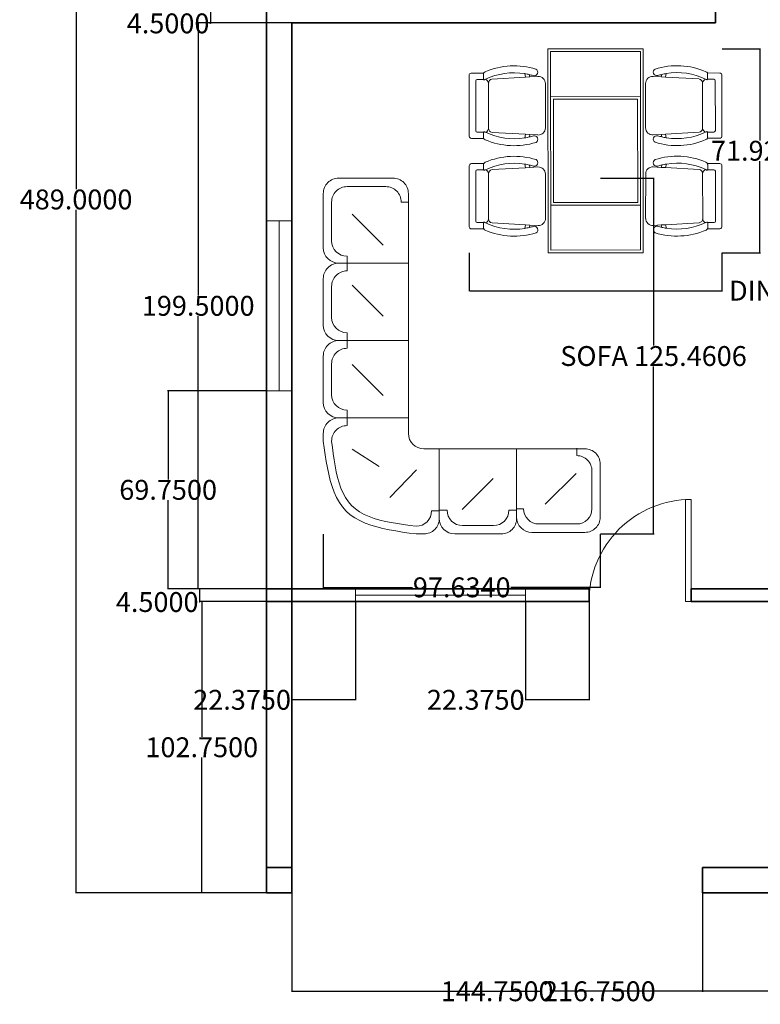
# Model space of a CAD drawing. Units: inches. Extents: x 774 to 2194, y 522 to 1247.
# Tile 1 of 7: x 774 to 1035, y 522 to 870. Entities that reach past the tile are written whole.
import ezdxf

# ---------------------------------------------------------------- set-up
doc = ezdxf.new("R2010")
doc.units = ezdxf.units.IN
for name, color, linetype, lineweight in [('A-ANNO-DIMS', 2, 'Continuous', 13), ('A-DOOR', 3, 'Continuous', 18), ('A-FURN', 8, 'Continuous', 18), ('A-GLAZ', 4, 'Continuous', 18), ('A-WALL', 7, 'Continuous', 35)]:
    doc.layers.add(name, color=color, linetype=linetype, lineweight=lineweight)
doc.styles.get("Standard").update_dxf_attribs({"font": 'arial.ttf'})
doc.dimstyles.get("Standard").update_dxf_attribs({"dimtxt": 7, "dimasz": 0.18, "dimexe": 0.18, "dimexo": 0.0625, "dimgap": 0.09, "dimtad": 0, "dimtih": 1, "dimtoh": 1, "dimdec": 4, "dimzin": 0, "dimdsep": 46, "dimtxsty": 'Standard', "dimcen": 0.09, "dimadec": 0, "dimazin": 0, "dimtfac": 1, "dimtdec": 4, "dimtofl": 0, "dimtmove": 0, "dimatfit": 3, "dimfxl": 1, "dimtolj": 1, "dimtzin": 0, "dimarcsym": 0})

# ---------------------------------------------------------------- blocks, each defined once
blk = doc.blocks.new('A$C7D96336B')
for p, q in [((280, 0.2), (-280, -0.2)), ((280.8, -1199.8), (280, 0.2)), ((-280, -0.2), (-279.2, -1200.2)), ((264, -15.8), (-264, -16.2)), ((-264, -16.2), (-263.2, -1184.2)), ((264.8, -1183.8), (264, -15.8)), ((-742.8, -515.1), (-743.2, -156.2)), ((-658.1, -143.4), (-730.7, -143.6)), ((-659.8, -143.4), (-659.7, -178.7)), ((-411.5, -167.3), (-609.1, -178.7)), ((-416.5, -146.3), (-411.5, -167.3)), ((-386.1, -165.8), (-411.5, -167.3)), ((-389.5, -151.7), (-386.1, -165.8)), ((-338.9, -163.1), (-386.1, -165.8)), ((339.1, -162.6), (386.3, -165.3)), ((389.7, -151.1), (386.3, -165.3)), ((386.3, -165.3), (411.7, -166.7)), ((416.7, -145.7), (411.7, -166.7)), ((411.7, -166.7), (609.3, -177.8)), ((658.3, -142.5), (730.9, -142.6)), ((659.9, -142.6), (659.9, -177.8)), ((743.5, -514.1), (743.4, -155.2)), ((-704.9, -188.8), (-704.6, -482.3)), ((-659.3, -180.3), (-696.6, -180.5)), ((-629.9, -467.6), (-630.2, -203.4)), ((-294.5, -465.7), (-294.4, -204.7)), ((295.2, -465.3), (294.7, -204.3)), ((630.5, -466.8), (630.5, -202.5)), ((659.5, -179.5), (696.9, -179.5)), ((705.2, -187.9), (705.3, -481.4)), ((-263.8, -280.2), (264.2, -279.8)), ((-263.8, -280.2), (264.2, -279.8)), ((-263.4, -920.2), (-263.8, -280.2)), ((264.2, -279.8), (264.6, -919.8)), ((-247.8, -296.2), (248.2, -295.8)), ((-247.4, -904.2), (-247.8, -296.2)), ((248.2, -295.8), (248.6, -903.8)), ((-659, -490.7), (-696.3, -490.7)), ((-659.4, -522.3), (-659.3, -492.4)), ((-411.1, -503.3), (-608.7, -492.3)), ((-416.1, -524.3), (-411.1, -503.3)), ((-385.8, -504.7), (-411.1, -503.3)), ((-389.1, -518.8), (-385.8, -504.7)), ((-338.5, -507.3), (-385.8, -504.7)), ((339.2, -506.9), (386.5, -504.2)), ((386.5, -504.2), (411.8, -502.7)), ((389.8, -518.3), (386.5, -504.2)), ((411.8, -502.7), (609.4, -491.4)), ((416.8, -523.7), (411.8, -502.7)), ((659.6, -489.8), (697, -489.7)), ((660.1, -521.4), (660, -491.5)), ((-657.7, -527.6), (-730.3, -527.6)), ((658.4, -526.7), (731, -526.6)), ((-742.7, -688.4), (-742.6, -1047.3)), ((-657.6, -675.8), (-730.2, -675.9)), ((-659.3, -681), (-659.2, -711)), ((-416, -678.8), (-411, -699.8)), ((-389, -684.2), (-385.6, -698.3)), ((339.3, -695.2), (386.6, -697.8)), ((389.9, -683.7), (386.6, -697.8)), ((416.9, -678.2), (411.9, -699.2)), ((658.5, -674.9), (731.1, -674.9)), ((660.2, -680.2), (660.2, -710.1)), ((743.6, -687.4), (744, -1046.3)), ((-704.4, -1014.6), (-704.5, -721.1)), ((-658.8, -712.7), (-696.2, -712.8)), ((-629.7, -735.7), (-629.6, -1000)), ((-411, -699.8), (-608.6, -711)), ((-385.6, -698.3), (-411, -699.8)), ((-338.4, -695.6), (-385.6, -698.3)), ((-294.4, -737.1), (-293.9, -998.2)), ((295.3, -736.7), (295.2, -997.8)), ((386.6, -697.8), (411.9, -699.2)), ((411.9, -699.2), (609.5, -710.2)), ((630.7, -734.9), (631, -999.1)), ((659.8, -711.8), (697.1, -711.8)), ((705.8, -1013.7), (705.5, -720.2)), ((264.6, -919.8), (-263.4, -920.2)), ((248.6, -903.8), (-247.4, -904.2)), ((-658.7, -1023), (-696.1, -1023)), ((-659.1, -1059.9), (-659.1, -1024.7)), ((-410.9, -1035.8), (-608.5, -1024.6)), ((-415.9, -1056.8), (-410.9, -1035.8)), ((-385.5, -1037.2), (-410.9, -1035.8)), ((-388.9, -1051.4), (-385.5, -1037.2)), ((-338.3, -1039.9), (-385.5, -1037.2)), ((339.7, -1039.4), (386.9, -1036.7)), ((386.9, -1036.7), (412.3, -1035.2)), ((390.3, -1050.8), (386.9, -1036.7)), ((412.3, -1035.2), (609.9, -1023.8)), ((417.3, -1056.2), (412.3, -1035.2)), ((660.1, -1022.1), (697.4, -1022)), ((660.6, -1059), (660.5, -1023.8)), ((-657.5, -1059.9), (-730.1, -1059.9)), ((658.9, -1059), (731.5, -1058.9)), ((-279.2, -1200.2), (280.8, -1199.8)), ((-263.2, -1184.2), (264.8, -1183.8))]:
    blk.add_line(p, q)
for centre, radius, start, end in [((-478.6, -532.7), 432.3, 72.71189, 113.32582), ((479.4, -532), 432.3, 66.7517, 107.36563), ((-730.7, -156.1), 12.5, 141.76048, 180.14594), ((-730.7, -156.1), 12.5, 90.1463, 141.76048), ((-643.2, -151), 16.7, 153.00405, 184.85665), ((-643.2, -151), 16.7, 113.32582, 153.00405), ((-479.1, -531.9), 390.7, 80.77031, 115.5809), ((-479.1, -531.9), 390.7, 76.73356, 80.77031), ((-479.1, -531.9), 390.7, 73.16759, 76.73356), ((-360.6, -137.9), 20.8, 254.77951, 60.01862), ((-336.5, -204.7), 41.7, 0.1463, 93.30684), ((336.7, -204.2), 41.7, 86.77068, 179.93121), ((360.7, -137.4), 20.8, 120.05889, 285.29801), ((479.9, -531.2), 390.7, 103.34395, 106.90992), ((479.9, -531.2), 390.7, 99.3072, 103.34395), ((479.9, -531.2), 390.7, 64.49661, 99.3072), ((643.4, -150.1), 16.7, 27.07347, 66.7517), ((643.4, -150.1), 16.7, 355.22086, 27.07347), ((730.9, -155.1), 12.5, 38.31704, 89.93121), ((730.9, -155.1), 12.5, 359.93158, 38.31704), ((-696.6, -188.8), 8.33, 90.1463, 180.1463), ((-655.5, -178.6), 4.17, 180.1463, 296.52957), ((-479.1, -531.9), 390.7, 115.5809, 116.52957), ((-655.2, -203.4), 25, 0.1463, 72.89681), ((-605.2, -203.4), 25, 98.92093, 179.97138), ((605.5, -202.6), 25, 0.10613, 81.15658), ((655.5, -202.5), 25, 107.1807, 179.93121), ((479.9, -531.2), 390.7, 63.54795, 64.49661), ((655.7, -177.8), 4.17, 243.54795, 359.93121), ((696.9, -187.8), 8.33, 359.93121, 89.93121), ((-730.3, -515.1), 12.5, 179.97174, 218.3572), ((-696.3, -482.3), 8.33, 179.97138, 269.97138), ((-642.9, -520), 16.7, 175.26103, 207.11363), ((-655.2, -492.4), 4.17, 63.58811, 179.97138), ((-479.5, -138.8), 390.7, 243.58811, 244.53678), ((-654.9, -467.6), 25, 287.22087, 359.97138), ((-479.5, -138.8), 390.7, 244.53678, 279.34737), ((-604.9, -467.6), 25, 180.1463, 261.19675), ((-479.5, -138.8), 390.7, 279.34737, 283.38411), ((-479.5, -138.8), 390.7, 283.38411, 286.95009), ((-360.2, -532.5), 20.8, 300.09905, 105.33817), ((-336.2, -465.7), 41.7, 266.81084, 359.97138), ((336.8, -465.3), 41.7, 180.10613, 273.26667), ((360.9, -532), 20.8, 74.73934, 239.97846), ((479.7, -138.1), 390.7, 253.12743, 256.6934), ((479.7, -138.1), 390.7, 256.6934, 260.73015), ((479.7, -138.1), 390.7, 260.73015, 295.54074), ((605.5, -466.7), 25, 278.88077, 359.93121), ((655.5, -466.7), 25, 180.10613, 252.85665), ((479.7, -138.1), 390.7, 295.54074, 296.4894), ((655.8, -491.5), 4.17, 0.10613, 116.4894), ((643.6, -519.1), 16.7, 332.96388, 4.81649), ((697, -481.4), 8.33, 270.10613, 0.10613), ((731, -514.1), 12.5, 321.72031, 0.10577), ((-730.3, -515.1), 12.5, 218.3572, 269.97138), ((-642.9, -520), 16.7, 207.11363, 246.79186), ((-479.1, -138), 432.3, 246.79186, 287.40579), ((479.2, -137.3), 432.3, 252.67172, 293.28565), ((643.6, -519.1), 16.7, 293.28565, 332.96388), ((731, -514.1), 12.5, 270.10613, 321.72031), ((-478.4, -1065.1), 432.3, 72.67172, 113.28565), ((479.9, -1064.5), 432.3, 66.79186, 107.40579), ((-730.2, -688.4), 12.5, 141.72031, 180.10577), ((-730.2, -688.4), 12.5, 90.10613, 141.72031), ((-642.7, -683.3), 16.7, 152.96388, 184.81649), ((-642.7, -683.3), 16.7, 113.28565, 152.96388), ((-478.9, -1064.3), 390.7, 80.73015, 115.54074), ((-478.9, -1064.3), 390.7, 76.6934, 80.73015), ((-478.9, -1064.3), 390.7, 73.12743, 76.6934), ((-360.1, -670.4), 20.8, 254.73934, 59.97846), ((337, -736.8), 41.7, 86.81084, 179.97138), ((361, -670), 20.8, 120.09905, 285.33817), ((480.4, -1063.7), 390.7, 103.38411, 106.95009), ((480.4, -1063.7), 390.7, 99.34737, 103.38411), ((480.4, -1063.7), 390.7, 64.53678, 99.34737), ((643.7, -682.5), 16.7, 27.11363, 66.79186), ((643.7, -682.5), 16.7, 355.26103, 27.11363), ((731.1, -687.4), 12.5, 38.3572, 89.97138), ((731.1, -687.4), 12.5, 359.97174, 38.3572), ((-696.1, -721.1), 8.33, 90.10613, 180.10613), ((-655, -711), 4.17, 180.10613, 296.4894), ((-478.9, -1064.3), 390.7, 115.54074, 116.4894), ((-654.7, -735.8), 25, 0.10613, 72.85665), ((-604.7, -735.7), 25, 98.88077, 179.93121), ((-336, -737.2), 41.7, 0.10613, 93.26667), ((605.7, -734.9), 25, 0.1463, 81.19675), ((655.7, -734.9), 25, 107.22087, 179.97138), ((480.4, -1063.7), 390.7, 63.58811, 64.53678), ((656, -710.1), 4.17, 243.58811, 359.97138), ((697.1, -720.1), 8.33, 359.97138, 89.97138), ((-696.1, -1014.6), 8.33, 179.93121, 269.93121), ((-654.9, -1024.7), 4.17, 63.54795, 179.93121), ((-479.1, -671.2), 390.7, 243.54795, 244.49661), ((-654.6, -1000), 25, 287.1807, 359.93121), ((-479.1, -671.2), 390.7, 244.49661, 279.3072), ((-604.6, -999.9), 25, 180.10613, 261.15658), ((-335.9, -998.3), 41.7, 266.77068, 359.93121), ((337.3, -997.8), 41.7, 180.1463, 273.30684), ((480, -670.6), 390.7, 260.77031, 295.5809), ((606, -999.1), 25, 278.92093, 359.97138), ((656, -999.1), 25, 180.1463, 252.89681), ((480, -670.6), 390.7, 295.5809, 296.52957), ((656.3, -1023.8), 4.17, 0.1463, 116.52957), ((697.4, -1013.7), 8.33, 270.1463, 0.1463), ((-730.1, -1047.4), 12.5, 179.93158, 218.31704), ((-730.1, -1047.4), 12.5, 218.31704, 269.93121), ((-642.6, -1052.4), 16.7, 175.22086, 207.07347), ((-642.6, -1052.4), 16.7, 207.07347, 246.7517), ((-478.6, -670.4), 432.3, 246.7517, 287.36563), ((-479.1, -671.2), 390.7, 279.3072, 283.34395), ((-479.1, -671.2), 390.7, 283.34395, 286.90992), ((-359.9, -1065.1), 20.8, 300.05889, 105.29801), ((361.4, -1064.6), 20.8, 74.77951, 240.01862), ((479.5, -669.8), 432.3, 252.71189, 293.32582), ((480, -670.6), 390.7, 253.16759, 256.73356), ((480, -670.6), 390.7, 256.73356, 260.77031), ((644, -1051.5), 16.7, 293.32582, 333.00405), ((644, -1051.5), 16.7, 333.00405, 4.85665), ((731.5, -1046.4), 12.5, 270.1463, 321.76048), ((731.5, -1046.4), 12.5, 321.76048, 0.14594)]:
    blk.add_arc(centre, radius, start, end)
blk = doc.blocks.new('A$C4B324E0D')
for points in [[(-0.4032, -0.0374), (-0.3959, 0.0153), (-0.3883, 0.0678), (-0.3801, 0.1195), (-0.3709, 0.1704), (-0.3605, 0.22), (-0.3485, 0.2679), (-0.3346, 0.314), (-0.3185, 0.3579), (-0.2998, 0.3993), (-0.2783, 0.4378), (-0.2537, 0.4731), (-0.2255, 0.5049), (-0.1936, 0.5331), (-0.1583, 0.5578), (-0.1198, 0.5793), (-0.0785, 0.5979), (-0.0346, 0.614), (0.0115, 0.628), (0.0595, 0.64), (0.1091, 0.6504), (0.1599, 0.6595), (0.2117, 0.6678), (0.2641, 0.6753), (0.3168, 0.6826)], [(-0.3432, -0.0374), (-0.3369, 0.0114), (-0.3303, 0.0599), (-0.3232, 0.1078), (-0.3151, 0.1548), (-0.3059, 0.2006), (-0.2951, 0.2449), (-0.2826, 0.2874), (-0.2681, 0.3278), (-0.2511, 0.3658), (-0.2315, 0.4011), (-0.2089, 0.4335), (-0.1831, 0.4625), (-0.1538, 0.488), (-0.1214, 0.5102), (-0.086, 0.5294), (-0.0479, 0.546), (-0.0075, 0.5602), (0.035, 0.5722), (0.0793, 0.5825), (0.125, 0.5914), (0.172, 0.599), (0.2198, 0.6057), (0.2682, 0.6119), (0.3168, 0.6177)], [(0.3768, 0.6826), (0.3168, 0.6826)], [(0.3168, 0.6177), (0.3168, 0.6177)], [(0.9768, 0.6826), (0.6168, 0.6826)], [(0.9168, 0.6177), (0.6768, 0.6177)], [(1.5769, 0.6826), (1.2168, 0.6826)], [(1.5168, 0.6177), (1.2768, 0.6177)], [(1.8168, 0.6826), (2.2368, 0.6826)], [(2.1704, 0.6177), (1.8704, 0.6177)], [(0.4968, 0.0226), (0.4968, 0.5626)], [(0.4968, 0.5626), (0.4968, 0.0226), (1.0968, 0.0226)], [(1.0968, 0.5626), (1.0968, 0.0226), (1.6968, 0.0226)], [(1.0968, 0.0226), (1.0968, 0.5626)], [(1.6968, 0.0226), (1.6968, 0.5626)], [(2.2368, 0.0226), (1.6968, 0.0226), (1.6968, 0.5626)], [(2.3569, 0.5626), (2.3569, 0.1426)], [(0.4968, 0.4977), (0.4368, 0.4977), (0.4368, 0.4977)], [(0.5569, 0.4977), (0.5569, 0.4977), (0.4968, 0.4977)], [(1.0968, 0.4977), (1.0368, 0.4977), (1.0368, 0.4977)], [(1.1569, 0.4977), (1.1569, 0.4977), (1.0968, 0.4977)], [(1.6969, 0.4977), (1.6368, 0.4977), (1.6368, 0.4977)], [(1.7504, 0.4977), (1.7504, 0.4977), (1.6904, 0.4977)], [(2.2904, 0.1977), (2.2904, 0.4977)], [(0.255, 0.4573), (0.1211, 0.2495)], [(0.9111, 0.4573), (0.6711, 0.2173)], [(1.527, 0.4573), (1.287, 0.2173)], [(2.0759, 0.4573), (1.8359, 0.2173)], [(-0.1199, 0.1664), (0.0943, -0.0414)], [(2.1704, 0.0177), (2.1704, 0.0777), (2.1704, 0.0777)], [(0.4968, 0.0226), (0.3768, 0.0226)], [(-0.4032, -0.0974), (-0.4032, -0.0374)], [(-0.3432, -0.0374), (-0.3432, -0.0374)], [(0.2568, -0.0974), (0.2568, -0.2174)], [(-0.2832, -0.8174), (0.2568, -0.8174), (0.2568, -0.2174)], [(0.2568, -0.2174), (-0.2832, -0.2174)], [(0.2568, -0.2174), (-0.2832, -0.2174)], [(-0.2232, -0.2174), (-0.2232, -0.1574), (-0.2232, -0.1574)], [(-0.2183, -0.2174), (-0.2183, -0.2774), (-0.2183, -0.2774)], [(-0.4032, -0.3374), (-0.4032, -0.6974)], [(-0.3383, -0.3974), (-0.3383, -0.6374)], [(-0.2136, -0.3946), (0.0264, -0.6346)], [(-0.2183, -0.7574), (-0.2183, -0.7574), (-0.2183, -0.8174)], [(0.2568, -0.8174), (-0.2832, -0.8174)], [(-0.2732, -0.8174), (0.2568, -0.8174), (0.2568, -1.3475)], [(-0.208, -0.8126), (-0.208, -0.8715), (-0.208, -0.8715)], [(0.2568, -0.8174), (0.2568, -1.3475)], [(-0.391, -1.3475), (-0.391, -0.9352)], [(-0.3258, -0.9893), (-0.3258, -1.2838)], [(-0.1734, -1.0387), (0.0666, -1.2787)], [(0.2043, -1.2838), (0.2043, -1.2838), (0.2632, -1.2838)], [(-0.208, -1.4016), (0.0865, -1.4016)], [(0.1391, -1.4653), (-0.2732, -1.4653)]]:
    blk.add_lwpolyline(points)
for centre, radius, start, end in [((0.3168, 0.4977), 0.12, 0, 90), ((0.3768, 0.5626), 0.12, 0, 90), ((0.6168, 0.5626), 0.12, 90, 180), ((0.6768, 0.4977), 0.12, 90, 180), ((0.9168, 0.4977), 0.12, 0, 90), ((0.9768, 0.5626), 0.12, 0, 90), ((1.2168, 0.5626), 0.12, 90, 180), ((1.2768, 0.4977), 0.12, 90, 180), ((1.5168, 0.4977), 0.12, 0, 90), ((1.5769, 0.5626), 0.12, 0, 90), ((1.8168, 0.5626), 0.12, 90, 180), ((1.8704, 0.4977), 0.12, 90, 180), ((2.1704, 0.4977), 0.12, 0, 90), ((2.2368, 0.5626), 0.12, 0, 90), ((2.1704, 0.1977), 0.12, 270, 0), ((2.2368, 0.1426), 0.12, 270, 0), ((0.3768, -0.0974), 0.12, 90, 180), ((-0.2232, -0.0374), 0.12, 180, 270), ((-0.2832, -0.0974), 0.12, 179.9997, 270), ((-0.2832, -0.3374), 0.12, 90, 180), ((-0.2183, -0.3974), 0.12, 90, 180), ((-0.2183, -0.6374), 0.12, 180, 270), ((-0.2832, -0.6974), 0.12, 179.9997, 270), ((-0.2732, -0.9352), 0.1178, 90, 180), ((-0.208, -0.9893), 0.1178, 90, 180), ((-0.208, -1.2838), 0.1178, 180, 270), ((0.0865, -1.2838), 0.1178, 270, 0), ((-0.2732, -1.3475), 0.1178, 179.9997, 270), ((0.1391, -1.3475), 0.1178, 270, 0)]:
    blk.add_arc(centre, radius, start, end)
blk = doc.blocks.new('A$C58C6152E')
at = {"xscale": 1.5, "yscale": 1.5, "zscale": 1.5, "rotation": 90}
blk.add_blockref('A$C4B324E0D', (1.024, 0.605), dxfattribs=at)
blk = doc.blocks.new('A$C15DC316E')
at = {"xscale": -1, "rotation": 270}
blk.add_blockref('A$C58C6152E', (0, 0), dxfattribs=at)
blk = doc.blocks.new('*D18')
at = {"layer": 'A-ANNO-DIMS', "color": 0, "lineweight": -2, "transparency": 16777216}
for p, q in [((869.72, 872.94), (840.87, 872.94)), ((841.05, 872.76), (841.05, 868.62)), ((869.72, 868.44), (840.87, 868.44)), ((841.05, 868.26), (840.87, 868.26)), ((841.05, 868.44), (841.05, 868.26))]:
    blk.add_line(p, q, dxfattribs=at)
at = {"layer": 'A-ANNO-DIMS', "color": 0, "transparency": 16777216}
for points in [[(841.02, 872.76), (841.08, 872.76), (841.05, 872.94)], [(841.02, 868.62), (841.08, 868.62), (841.05, 868.44)]]:
    blk.add_solid(points, dxfattribs=at)
at = {"layer": 'Defpoints', "color": 0, "transparency": 16777216}
for p in [(869.78, 872.94), (841.05, 868.44), (869.78, 868.44)]:
    blk.add_point(p, dxfattribs=at)
at = {"layer": 'A-ANNO-DIMS', "color": 0, "transparency": 16777216, "insert": (826.12, 868.26), "char_height": 7, "attachment_point": 5}
blk.add_mtext('\\A1;4.5000', dxfattribs=at)
blk = doc.blocks.new('*D19')
at = {"layer": 'A-ANNO-DIMS', "color": 0, "lineweight": -2, "transparency": 16777216}
for p, q in [((869.72, 868.44), (836.55, 868.44)), ((836.73, 868.26), (836.73, 772.35)), ((836.73, 669.12), (836.73, 765.02)), ((869.72, 668.94), (836.55, 668.94))]:
    blk.add_line(p, q, dxfattribs=at)
at = {"layer": 'A-ANNO-DIMS', "color": 0, "transparency": 16777216}
for points in [[(836.7, 868.26), (836.76, 868.26), (836.73, 868.44)], [(836.7, 669.12), (836.76, 669.12), (836.73, 668.94)]]:
    blk.add_solid(points, dxfattribs=at)
at = {"layer": 'Defpoints', "color": 0, "transparency": 16777216}
for p in [(869.78, 868.44), (836.73, 668.94), (869.78, 668.94)]:
    blk.add_point(p, dxfattribs=at)
at = {"layer": 'A-ANNO-DIMS', "color": 0, "transparency": 16777216, "insert": (836.73, 768.69), "char_height": 7, "attachment_point": 5}
blk.add_mtext('\\A1;199.5000', dxfattribs=at)
blk = doc.blocks.new('*D20')
at = {"layer": 'A-ANNO-DIMS', "color": 0, "lineweight": -2, "transparency": 16777216}
for p, q in [((869.72, 668.94), (837.03, 668.94)), ((837.21, 668.76), (837.21, 664.62)), ((869.72, 664.44), (837.03, 664.44)), ((837.21, 664.26), (837.03, 664.26)), ((837.21, 664.44), (837.21, 664.26))]:
    blk.add_line(p, q, dxfattribs=at)
at = {"layer": 'A-ANNO-DIMS', "color": 0, "transparency": 16777216}
for points in [[(837.18, 668.76), (837.24, 668.76), (837.21, 668.94)], [(837.18, 664.62), (837.24, 664.62), (837.21, 664.44)]]:
    blk.add_solid(points, dxfattribs=at)
at = {"layer": 'Defpoints', "color": 0, "transparency": 16777216}
for p in [(869.78, 668.94), (837.21, 664.44), (869.78, 664.44)]:
    blk.add_point(p, dxfattribs=at)
at = {"layer": 'A-ANNO-DIMS', "color": 0, "transparency": 16777216, "insert": (822.28, 664.26), "char_height": 7, "attachment_point": 5}
blk.add_mtext('\\A1;4.5000', dxfattribs=at)
blk = doc.blocks.new('*D21')
at = {"layer": 'A-ANNO-DIMS', "color": 0, "lineweight": -2, "transparency": 16777216}
for p, q in [((869.72, 664.44), (837.82, 664.44)), ((838, 664.26), (838, 616.73)), ((838, 561.87), (838, 609.4)), ((869.72, 561.69), (837.82, 561.69))]:
    blk.add_line(p, q, dxfattribs=at)
at = {"layer": 'A-ANNO-DIMS', "color": 0, "transparency": 16777216}
for points in [[(837.97, 664.26), (838.03, 664.26), (838, 664.44)], [(837.97, 561.87), (838.03, 561.87), (838, 561.69)]]:
    blk.add_solid(points, dxfattribs=at)
at = {"layer": 'Defpoints', "color": 0, "transparency": 16777216}
for p in [(869.78, 664.44), (838, 561.69), (869.78, 561.69)]:
    blk.add_point(p, dxfattribs=at)
at = {"layer": 'A-ANNO-DIMS', "color": 0, "transparency": 16777216, "insert": (838, 613.06), "char_height": 7, "attachment_point": 5}
blk.add_mtext('\\A1;102.7500', dxfattribs=at)
blk = doc.blocks.new('*D22')
at = {"layer": 'A-ANNO-DIMS', "color": 0, "lineweight": -2, "transparency": 16777216}
for p, q in [((869.72, 1050.69), (793.49, 1050.69)), ((793.67, 1050.51), (793.67, 809.85)), ((793.67, 561.87), (793.67, 802.52)), ((869.72, 561.69), (793.49, 561.69))]:
    blk.add_line(p, q, dxfattribs=at)
at = {"layer": 'A-ANNO-DIMS', "color": 0, "transparency": 16777216}
for points in [[(793.64, 1050.51), (793.7, 1050.51), (793.67, 1050.69)], [(793.64, 561.87), (793.7, 561.87), (793.67, 561.69)]]:
    blk.add_solid(points, dxfattribs=at)
at = {"layer": 'Defpoints', "color": 0, "transparency": 16777216}
for p in [(869.78, 1050.69), (793.67, 561.69), (869.78, 561.69)]:
    blk.add_point(p, dxfattribs=at)
at = {"layer": 'A-ANNO-DIMS', "color": 0, "transparency": 16777216, "insert": (793.67, 806.19), "char_height": 7, "attachment_point": 5}
blk.add_mtext('\\A1;489.0000', dxfattribs=at)
blk = doc.blocks.new('DOOR-SWING-36IN')
blk.add_line((36, 0), (36, 2))
blk.add_lwpolyline([(36, 2), (0, 2), (0, 0), (36, 0)], close=True)
blk.add_arc((36, 0), 36, 90, 180)
blk = doc.blocks.new('WIN-60IN-EXT')
for p, q in [((0, 0), (0, 9)), ((60, 0), (60, 9)), ((0, 4.5), (60, 4.5))]:
    blk.add_line(p, q)
blk = doc.blocks.new('*D46')
at = {"layer": 'A-ANNO-DIMS', "color": 0, "lineweight": -2, "transparency": 16777216}
for p, q in [((932.28, 787.34), (932.28, 773.85)), ((1021.39, 787.34), (1021.39, 773.85)), ((932.46, 774.03), (1021.21, 774.03)), ((1021.39, 774.03), (1021.57, 774.03))]:
    blk.add_line(p, q, dxfattribs=at)
at = {"layer": 'A-ANNO-DIMS', "color": 0, "transparency": 16777216}
for points in [[(932.46, 774.06), (932.46, 774), (932.28, 774.03)], [(1021.21, 774.06), (1021.21, 774), (1021.39, 774.03)]]:
    blk.add_solid(points, dxfattribs=at)
at = {"layer": 'Defpoints', "color": 0, "transparency": 16777216}
for p in [(932.28, 787.4), (1021.39, 787.4), (1021.39, 774.03)]:
    blk.add_point(p, dxfattribs=at)
at = {"layer": 'A-ANNO-DIMS', "color": 0, "transparency": 16777216, "insert": (1068.06, 774.03), "char_height": 7, "attachment_point": 5}
blk.add_mtext('\\A1;DINING SET 89.1080', dxfattribs=at)
blk = doc.blocks.new('*D47')
at = {"layer": 'A-ANNO-DIMS', "color": 0, "lineweight": -2, "transparency": 16777216}
for p, q in [((1021.45, 859.32), (1034.94, 859.32)), ((1034.76, 859.14), (1034.76, 827.02)), ((1034.76, 787.58), (1034.76, 819.7)), ((1021.45, 787.4), (1034.94, 787.4))]:
    blk.add_line(p, q, dxfattribs=at)
at = {"layer": 'A-ANNO-DIMS', "color": 0, "transparency": 16777216}
for points in [[(1034.73, 859.14), (1034.79, 859.14), (1034.76, 859.32)], [(1034.73, 787.58), (1034.79, 787.58), (1034.76, 787.4)]]:
    blk.add_solid(points, dxfattribs=at)
at = {"layer": 'Defpoints', "color": 0, "transparency": 16777216}
for p in [(1021.39, 859.32), (1034.76, 859.32), (1021.39, 787.4)]:
    blk.add_point(p, dxfattribs=at)
at = {"layer": 'A-ANNO-DIMS', "color": 0, "transparency": 16777216, "insert": (1034.76, 823.36), "char_height": 7, "attachment_point": 5}
blk.add_mtext('\\A1;71.9216', dxfattribs=at)
blk = doc.blocks.new('*D48')
at = {"layer": 'A-ANNO-DIMS', "color": 0, "lineweight": -2, "transparency": 16777216}
for p, q in [((978.53, 813.72), (997.46, 813.72)), ((997.28, 813.54), (997.28, 754.7)), ((997.28, 688.44), (997.28, 747.27)), ((978.53, 688.26), (997.46, 688.26))]:
    blk.add_line(p, q, dxfattribs=at)
at = {"layer": 'A-ANNO-DIMS', "color": 0, "transparency": 16777216}
for points in [[(997.25, 813.54), (997.31, 813.54), (997.28, 813.72)], [(997.25, 688.44), (997.31, 688.44), (997.28, 688.26)]]:
    blk.add_solid(points, dxfattribs=at)
at = {"layer": 'Defpoints', "color": 0, "transparency": 16777216}
for p in [(978.46, 813.72), (997.28, 813.72), (978.46, 688.26)]:
    blk.add_point(p, dxfattribs=at)
at = {"layer": 'A-ANNO-DIMS', "color": 0, "transparency": 16777216, "insert": (997.28, 750.99), "char_height": 7, "attachment_point": 5}
blk.add_mtext('\\A1;SOFA 125.4606', dxfattribs=at)
blk = doc.blocks.new('*D49')
at = {"layer": 'A-ANNO-DIMS', "color": 0, "lineweight": -2, "transparency": 16777216}
for p, q in [((880.83, 688.19), (880.83, 669.26)), ((978.46, 688.19), (978.46, 669.26)), ((881.01, 669.44), (912.32, 669.44)), ((978.28, 669.44), (946.97, 669.44))]:
    blk.add_line(p, q, dxfattribs=at)
at = {"layer": 'A-ANNO-DIMS', "color": 0, "transparency": 16777216}
for points in [[(881.01, 669.47), (881.01, 669.41), (880.83, 669.44)], [(978.28, 669.47), (978.28, 669.41), (978.46, 669.44)]]:
    blk.add_solid(points, dxfattribs=at)
at = {"layer": 'Defpoints', "color": 0, "transparency": 16777216}
for p in [(880.83, 688.26), (978.46, 688.26), (978.46, 669.44)]:
    blk.add_point(p, dxfattribs=at)
at = {"layer": 'A-ANNO-DIMS', "color": 0, "transparency": 16777216, "insert": (929.65, 669.44), "char_height": 7, "attachment_point": 5}
blk.add_mtext('\\A1;97.6340', dxfattribs=at)
blk = doc.blocks.new('*D54')
at = {"layer": 'A-ANNO-DIMS', "color": 0, "lineweight": -2, "transparency": 16777216}
for p, q in [((869.78, 561.63), (869.78, 526.86)), ((1014.53, 561.63), (1014.53, 526.86)), ((869.96, 527.04), (922.44, 527.04)), ((1014.35, 527.04), (961.87, 527.04))]:
    blk.add_line(p, q, dxfattribs=at)
at = {"layer": 'A-ANNO-DIMS', "color": 0, "transparency": 16777216}
for points in [[(869.96, 527.07), (869.96, 527.01), (869.78, 527.04)], [(1014.35, 527.07), (1014.35, 527.01), (1014.53, 527.04)]]:
    blk.add_solid(points, dxfattribs=at)
at = {"layer": 'Defpoints', "color": 0, "transparency": 16777216}
for p in [(869.78, 561.69), (1014.53, 561.69), (1014.53, 527.04)]:
    blk.add_point(p, dxfattribs=at)
at = {"layer": 'A-ANNO-DIMS', "color": 0, "transparency": 16777216, "insert": (942.16, 527.04), "char_height": 7, "attachment_point": 5}
blk.add_mtext('\\A1;144.7500', dxfattribs=at)
blk = doc.blocks.new('*D55')
at = {"layer": 'A-ANNO-DIMS', "color": 0, "lineweight": -2, "transparency": 16777216}
for p, q in [((869.78, 668.88), (869.78, 526.86)), ((1086.53, 668.88), (1086.53, 526.86)), ((869.96, 527.04), (958.05, 527.04)), ((1086.35, 527.04), (998.26, 527.04))]:
    blk.add_line(p, q, dxfattribs=at)
at = {"layer": 'A-ANNO-DIMS', "color": 0, "transparency": 16777216}
for points in [[(869.96, 527.07), (869.96, 527.01), (869.78, 527.04)], [(1086.35, 527.07), (1086.35, 527.01), (1086.53, 527.04)]]:
    blk.add_solid(points, dxfattribs=at)
at = {"layer": 'Defpoints', "color": 0, "transparency": 16777216}
for p in [(869.78, 668.94), (1086.53, 668.94), (1086.53, 527.04)]:
    blk.add_point(p, dxfattribs=at)
at = {"layer": 'A-ANNO-DIMS', "color": 0, "transparency": 16777216, "insert": (978.16, 527.04), "char_height": 7, "attachment_point": 5}
blk.add_mtext('\\A1;216.7500', dxfattribs=at)
blk = doc.blocks.new('*D56')
at = {"layer": 'A-ANNO-DIMS', "color": 0, "lineweight": -2, "transparency": 16777216}
for p, q in [((869.78, 664.38), (869.78, 629.61)), ((892.16, 664.38), (892.16, 629.61)), ((869.78, 629.79), (869.6, 629.79)), ((891.98, 629.79), (869.96, 629.79))]:
    blk.add_line(p, q, dxfattribs=at)
at = {"layer": 'A-ANNO-DIMS', "color": 0, "transparency": 16777216}
for points in [[(869.96, 629.82), (869.96, 629.76), (869.78, 629.79)], [(891.98, 629.82), (891.98, 629.76), (892.16, 629.79)]]:
    blk.add_solid(points, dxfattribs=at)
at = {"layer": 'Defpoints', "color": 0, "transparency": 16777216}
for p in [(869.78, 664.44), (892.16, 664.44), (869.78, 629.79)]:
    blk.add_point(p, dxfattribs=at)
at = {"layer": 'A-ANNO-DIMS', "color": 0, "transparency": 16777216, "insert": (852.21, 629.79), "char_height": 7, "attachment_point": 5}
blk.add_mtext('\\A1;22.3750', dxfattribs=at)
blk = doc.blocks.new('*D57')
at = {"layer": 'A-ANNO-DIMS', "color": 0, "lineweight": -2, "transparency": 16777216}
for p, q in [((952.16, 664.38), (952.16, 629.61)), ((974.53, 664.38), (974.53, 629.61)), ((952.16, 629.79), (951.98, 629.79)), ((974.35, 629.79), (952.34, 629.79))]:
    blk.add_line(p, q, dxfattribs=at)
at = {"layer": 'A-ANNO-DIMS', "color": 0, "transparency": 16777216}
for points in [[(952.34, 629.82), (952.34, 629.76), (952.16, 629.79)], [(974.35, 629.82), (974.35, 629.76), (974.53, 629.79)]]:
    blk.add_solid(points, dxfattribs=at)
at = {"layer": 'Defpoints', "color": 0, "transparency": 16777216}
for p in [(952.16, 664.44), (974.53, 664.44), (952.16, 629.79)]:
    blk.add_point(p, dxfattribs=at)
at = {"layer": 'A-ANNO-DIMS', "color": 0, "transparency": 16777216, "insert": (934.59, 629.79), "char_height": 7, "attachment_point": 5}
blk.add_mtext('\\A1;22.3750', dxfattribs=at)
blk = doc.blocks.new('*D62')
at = {"layer": 'A-ANNO-DIMS', "color": 0, "lineweight": -2, "transparency": 16777216}
for p, q in [((860.72, 738.69), (825.95, 738.69)), ((826.13, 738.51), (826.13, 707.48)), ((826.13, 669.12), (826.13, 700.15)), ((860.72, 668.94), (825.95, 668.94))]:
    blk.add_line(p, q, dxfattribs=at)
at = {"layer": 'A-ANNO-DIMS', "color": 0, "transparency": 16777216}
for points in [[(826.1, 738.51), (826.16, 738.51), (826.13, 738.69)], [(826.1, 669.12), (826.16, 669.12), (826.13, 668.94)]]:
    blk.add_solid(points, dxfattribs=at)
at = {"layer": 'Defpoints', "color": 0, "transparency": 16777216}
for p in [(826.13, 738.69), (860.78, 738.69), (860.78, 668.94)]:
    blk.add_point(p, dxfattribs=at)
at = {"layer": 'A-ANNO-DIMS', "color": 0, "transparency": 16777216, "insert": (826.13, 703.81), "char_height": 7, "attachment_point": 5}
blk.add_mtext('\\A1;69.7500', dxfattribs=at)

msp = doc.modelspace()

# ---------------------------------------------------------------- linework, layer by layer
at = {"layer": 'A-GLAZ'}
for p, q in [((892.15603, 664.4375), (892.15603, 668.9375)), ((892.15603, 666.6875), (952.15603, 666.6875)), ((952.15603, 664.4375), (952.15603, 668.9375))]:
    msp.add_line(p, q, dxfattribs=at)
at = {"layer": 'A-WALL'}
for p, q in [((860.78103, 1050.6875), (860.78103, 561.6875)), ((1019.07934, 872.9375), (1019.08056, 868.4375)), ((869.78103, 868.4375), (1019.08056, 868.4375)), ((869.78103, 868.4375), (869.78103, 668.9375)), ((869.78103, 868.4375), (869.78103, 561.6875)), ((860.78103, 668.9375), (974.53103, 668.9375)), ((974.53103, 664.4375), (974.53103, 668.9375)), ((1010.53103, 664.4375), (1010.53103, 668.9375)), ((1010.53103, 668.9375), (1086.53103, 668.9375)), ((860.78103, 664.4375), (974.53103, 664.4375)), ((869.78103, 664.4375), (974.53103, 664.4375)), ((1010.53103, 664.4375), (1211.78103, 664.4375)), ((860.78103, 570.6875), (869.78103, 570.6875)), ((1014.53103, 570.6875), (1014.53103, 561.6875)), ((1014.53103, 570.6875), (1211.78103, 570.6875)), ((860.78103, 561.6875), (869.78103, 561.6875)), ((1014.53103, 561.6875), (1220.78103, 561.6875))]:
    msp.add_line(p, q, dxfattribs=at)

# ---------------------------------------------------------------- block references
at = {"layer": 'A-DOOR', "extrusion": (0, 0, -1), "zscale": -1, "rotation": 270.0000000000003}
msp.add_blockref('DOOR-SWING-36IN', (-1010.53061, 700.43708), dxfattribs=at)
at = {"layer": 'A-FURN', "xscale": 0.0599157891524393, "yscale": 0.0599157891524393, "zscale": 0.0599157891524393}
msp.add_blockref('A$C7D96336B', (976.81224, 859.30902), dxfattribs=at)
at = {"layer": 'A-FURN', "xscale": -30.30437697783735, "yscale": 30.30437697783735, "zscale": 30.30437697783735, "rotation": 270}
msp.add_blockref('A$C15DC316E', (880.82882, 688.25576), dxfattribs=at)
at = {"layer": 'A-GLAZ', "rotation": 89.99999999999957}
msp.add_blockref('WIN-60IN-EXT', (869.78053, 738.68748), dxfattribs=at)

# ---------------------------------------------------------------- dimensions: what is measured, and where the dimension line sits
at = {"layer": 'A-ANNO-DIMS'}
for base, p1, p2, angle, override, picture, middle in [((793.67062, 561.6875), (869.78103, 1050.6875), (869.78103, 561.6875), 90, {"dimclrd": 0, "dimclre": 0, "dimclrt": 0}, '*D22', (793.67062, 806.1875)), ((841.05064, 868.4375), (869.78103, 872.9375), (869.78103, 868.4375), 90, {"dimclrd": 0, "dimclre": 0, "dimclrt": 0}, '*D18', (826.1217, 868.2575)), ((836.72755, 668.9375), (869.78103, 868.4375), (869.78103, 668.9375), 90, {"dimclrd": 0, "dimclre": 0, "dimclrt": 0}, '*D19', (836.72755, 768.6875)), ((1034.75683, 859.32037), (1021.39063, 787.39874), (1021.39063, 859.32037), 90, {"dimdec": 4, "dimlfac": 1, "dimrnd": 0, "dimzin": 0, "dimdsep": 46, "dimlunit": 2}, '*D47', (1034.75683, 823.35956)), ((826.13103, 738.6875), (860.78103, 668.9375), (860.78103, 738.6875), 90, {"dimdec": 4, "dimlfac": 1, "dimrnd": 0, "dimzin": 0, "dimdsep": 46, "dimlunit": 2}, '*D62', (826.13103, 703.8125)), ((837.20822, 664.4375), (869.78103, 668.9375), (869.78103, 664.4375), 90, {"dimclrd": 0, "dimclre": 0, "dimclrt": 0}, '*D20', (822.27928, 664.2575)), ((838.00015, 561.6875), (869.78103, 664.4375), (869.78103, 561.6875), 90, {"dimclrd": 0, "dimclre": 0, "dimclrt": 0}, '*D21', (838.00015, 613.0625)), ((869.78103, 629.7875), (892.15603, 664.4375), (869.78103, 664.4375), 180, {"dimdec": 4, "dimlfac": 1, "dimrnd": 0, "dimzin": 0, "dimdsep": 46, "dimlunit": 2}, '*D56', (852.21396, 629.7875)), ((952.15603, 629.7875), (974.53103, 664.4375), (952.15603, 664.4375), 180, {"dimdec": 4, "dimlfac": 1, "dimrnd": 0, "dimzin": 0, "dimdsep": 46, "dimlunit": 2}, '*D57', (934.58896, 629.7875))]:
    dim = msp.add_linear_dim(base=base, p1=p1, p2=p2, angle=angle, dimstyle='Standard', override=override, dxfattribs=at)
    dim.commit()
    dim.dimension.update_dxf_attribs({"geometry": picture, "text_midpoint": middle})
dim = msp.add_linear_dim(base=(997.28187, 813.71633), p1=(978.46278, 688.25575), p2=(978.46278, 813.71633), angle=90, text='SOFA <>', dimstyle='Standard', override={"dimdec": 4, "dimlfac": 1, "dimrnd": 0, "dimzin": 0, "dimdsep": 46, "dimlunit": 2}, dxfattribs=at)
dim.commit()
dim.dimension.update_dxf_attribs({"geometry": '*D48', "text_midpoint": (997.28187, 750.98604)})
dim = msp.add_linear_dim(base=(1021.39063, 774.03254), p1=(932.2826, 787.39874), p2=(1021.39063, 787.39874), text='DINING SET <>', dimstyle='Standard', override={"dimdec": 4, "dimlfac": 1, "dimrnd": 0, "dimzin": 0, "dimdsep": 46, "dimlunit": 2}, dxfattribs=at)
dim.commit()
dim.dimension.update_dxf_attribs({"geometry": '*D46', "text_midpoint": (1068.06308, 774.03254)})
for base, p1, p2, picture, middle in [((978.462781, 669.436669), (880.828825, 688.255755), (978.462781, 688.255755), '*D49', (929.645803, 669.436669)), ((1086.53103, 527.0375), (869.78103, 668.9375), (1086.53103, 668.9375), '*D55', (978.15603, 527.0375)), ((1014.53103, 527.0375), (869.78103, 561.6875), (1014.53103, 561.6875), '*D54', (942.15603, 527.0375))]:
    dim = msp.add_linear_dim(base=base, p1=p1, p2=p2, dimstyle='Standard', override={"dimdec": 4, "dimlfac": 1, "dimrnd": 0, "dimzin": 0, "dimdsep": 46, "dimlunit": 2}, dxfattribs=at)
    dim.commit()
    dim.dimension.update_dxf_attribs({"geometry": picture, "text_midpoint": middle})

doc.saveas('drawing.dxf')
